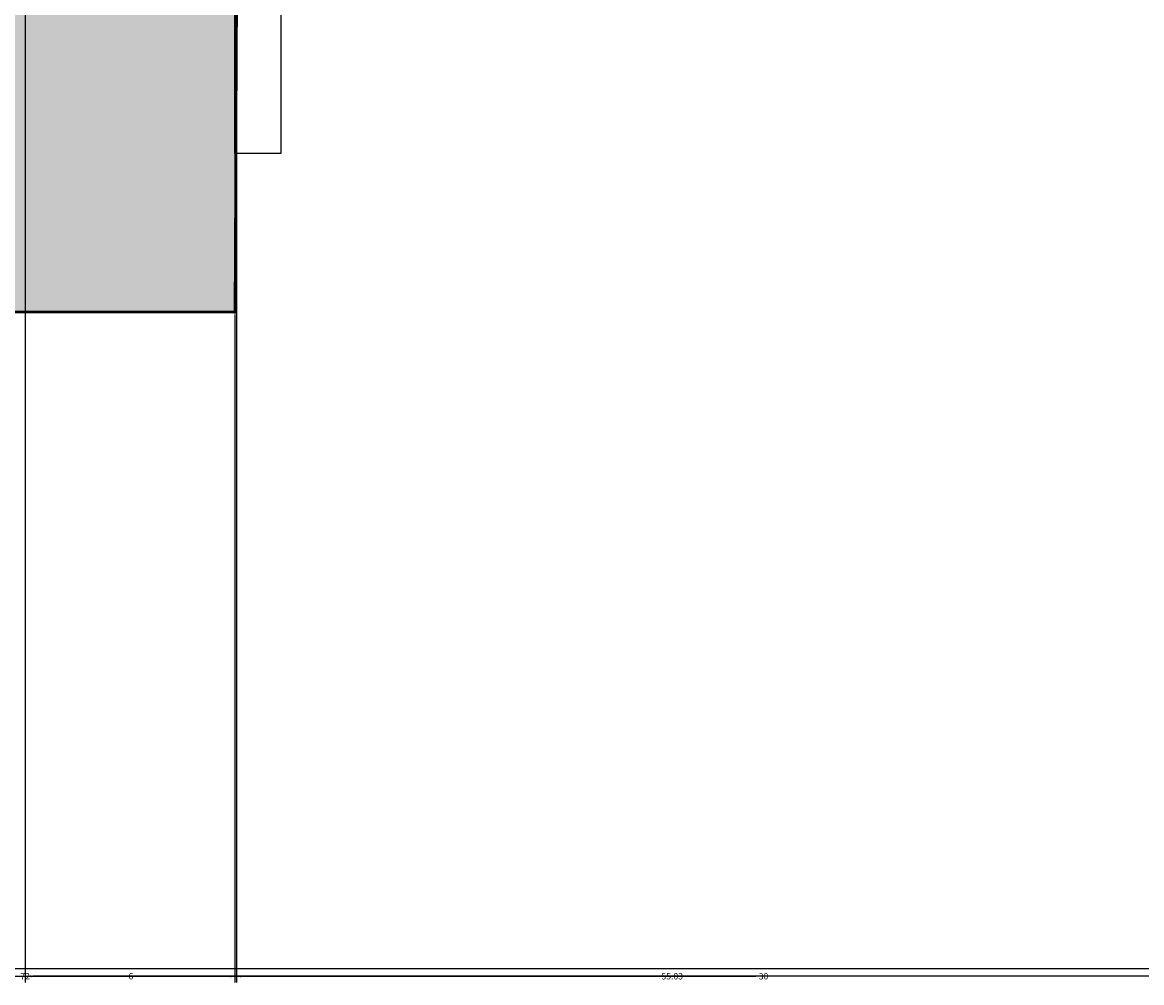
# Model space of a CAD drawing. Units: inches. Extents: x 2231 to 2461, y 2045 to 2455.
# Tile 4 of 95: x 2295 to 2326, y 2045 to 2072. Entities that reach past the tile are written whole.
import ezdxf

# ---------------------------------------------------------------- set-up
doc = ezdxf.new("R2010")
doc.units = ezdxf.units.IN
for name, color, linetype, lineweight in [('A-ANNO-DIMS', 2, 'Continuous', 18), ('A-DOOR', 3, 'Continuous', 25), ('A-WALL', 7, 'Continuous', 50)]:
    doc.layers.add(name, color=color, linetype=linetype, lineweight=lineweight)
doc.layers.add('A-WALL-PATT', color=18, linetype='Continuous', lineweight=13, true_color=0x000000)
doc.styles.get("Standard").update_dxf_attribs({"font": 'arial.ttf'})
doc.dimstyles.get("Standard").update_dxf_attribs({"dimtxt": 0.18, "dimasz": 0.18, "dimexe": 0.18, "dimexo": 0.0625, "dimgap": 0.09, "dimtad": 0, "dimtih": 1, "dimtoh": 1, "dimdec": 4, "dimzin": 0, "dimdsep": 46, "dimtxsty": 'Standard', "dimcen": 0.09, "dimadec": 0, "dimazin": 0, "dimtfac": 1, "dimtdec": 4, "dimtofl": 0, "dimtmove": 0, "dimatfit": 3, "dimfxl": 1, "dimtolj": 1, "dimtzin": 0, "dimarcsym": 0})

# ---------------------------------------------------------------- blocks, each defined once
blk = doc.blocks.new('*U5')
blk.add_line((0, 0), (0, -6))
blk.add_lwpolyline([(0, 0), (0, 40), (1.75, 40), (1.75, 0)], close=True)
blk.add_arc((0, 0), 40, 0, 90)
blk = doc.blocks.new('*D33')
at = {"layer": 'A-ANNO-DIMS', "color": 0, "lineweight": -2, "transparency": 16777216}
for p, q in [((2249.794, 2063.77), (2249.794, 2045.02)), ((2441.794, 2063.77), (2441.794, 2045.02)), ((2249.974, 2045.2), (2345.514, 2045.2)), ((2441.614, 2045.2), (2346.073, 2045.2))]:
    blk.add_line(p, q, dxfattribs=at)
at = {"layer": 'A-ANNO-DIMS', "color": 0, "transparency": 16777216}
for points in [[(2249.974, 2045.23), (2249.974, 2045.17), (2249.794, 2045.2)], [(2441.614, 2045.23), (2441.614, 2045.17), (2441.794, 2045.2)]]:
    blk.add_solid(points, dxfattribs=at)
at = {"layer": 'Defpoints', "color": 0, "transparency": 16777216}
for p in [(2249.794, 2063.833), (2441.794, 2063.833), (2249.794, 2045.2)]:
    blk.add_point(p, dxfattribs=at)
at = {"layer": 'A-ANNO-DIMS', "color": 0, "transparency": 16777216, "insert": (2345.794, 2045.2), "char_height": 0.18, "attachment_point": 5}
blk.add_mtext('\\A1;192', dxfattribs=at)
blk = doc.blocks.new('*D44')
at = {"layer": 'A-ANNO-DIMS', "color": 0, "lineweight": -2, "transparency": 16777216}
for p, q in [((2294.794, 2072.77), (2294.794, 2044.803)), ((2300.794, 2072.77), (2300.794, 2044.803)), ((2294.974, 2044.983), (2297.644, 2044.983)), ((2300.614, 2044.983), (2297.943, 2044.983))]:
    blk.add_line(p, q, dxfattribs=at)
at = {"layer": 'A-ANNO-DIMS', "color": 0, "transparency": 16777216}
for points in [[(2294.974, 2045.013), (2294.974, 2044.953), (2294.794, 2044.983)], [(2300.614, 2045.013), (2300.614, 2044.953), (2300.794, 2044.983)]]:
    blk.add_solid(points, dxfattribs=at)
at = {"layer": 'Defpoints', "color": 0, "transparency": 16777216}
for p in [(2294.794, 2072.833), (2300.794, 2072.833), (2300.794, 2044.983)]:
    blk.add_point(p, dxfattribs=at)
at = {"layer": 'A-ANNO-DIMS', "color": 0, "transparency": 16777216, "insert": (2297.794, 2044.983), "char_height": 0.18, "attachment_point": 5}
blk.add_mtext('\\A1;6', dxfattribs=at)
blk = doc.blocks.new('*D45')
at = {"layer": 'A-ANNO-DIMS', "color": 0, "lineweight": -2, "transparency": 16777216}
for p, q in [((2300.739, 2063.77), (2300.739, 2044.803)), ((2330.74, 2063.77), (2330.74, 2044.803)), ((2300.919, 2044.983), (2315.521, 2044.983)), ((2330.56, 2044.983), (2315.958, 2044.983))]:
    blk.add_line(p, q, dxfattribs=at)
at = {"layer": 'A-ANNO-DIMS', "color": 0, "transparency": 16777216}
for points in [[(2300.919, 2045.013), (2300.919, 2044.953), (2300.739, 2044.983)], [(2330.56, 2045.013), (2330.56, 2044.953), (2330.74, 2044.983)]]:
    blk.add_solid(points, dxfattribs=at)
at = {"layer": 'Defpoints', "color": 0, "transparency": 16777216}
for p in [(2300.739, 2063.833), (2330.74, 2063.833), (2330.74, 2044.983)]:
    blk.add_point(p, dxfattribs=at)
at = {"layer": 'A-ANNO-DIMS', "color": 0, "transparency": 16777216, "insert": (2315.739, 2044.983), "char_height": 0.18, "attachment_point": 5}
blk.add_mtext('\\A1;30', dxfattribs=at)
blk = doc.blocks.new('*D51')
at = {"layer": 'A-ANNO-DIMS', "color": 0, "lineweight": -2, "transparency": 16777216}
for p, q in [((2258.794, 2306.77), (2258.794, 2044.803)), ((2330.794, 2306.77), (2330.794, 2044.803)), ((2258.974, 2044.983), (2294.576, 2044.983)), ((2330.614, 2044.983), (2295.011, 2044.983))]:
    blk.add_line(p, q, dxfattribs=at)
at = {"layer": 'A-ANNO-DIMS', "color": 0, "transparency": 16777216}
for points in [[(2258.974, 2045.013), (2258.974, 2044.953), (2258.794, 2044.983)], [(2330.614, 2045.013), (2330.614, 2044.953), (2330.794, 2044.983)]]:
    blk.add_solid(points, dxfattribs=at)
at = {"layer": 'Defpoints', "color": 0, "transparency": 16777216}
for p in [(2258.794, 2306.833), (2330.794, 2306.833), (2330.794, 2044.983)]:
    blk.add_point(p, dxfattribs=at)
at = {"layer": 'A-ANNO-DIMS', "color": 0, "transparency": 16777216, "insert": (2294.794, 2044.983), "char_height": 0.18, "attachment_point": 5}
blk.add_mtext('\\A1;72', dxfattribs=at)
blk = doc.blocks.new('*D65')
at = {"layer": 'A-ANNO-DIMS', "color": 0, "lineweight": -2, "transparency": 16777216}
for p, q in [((2285.635, 2189.285), (2285.635, 2044.803)), ((2340.667, 2189.285), (2340.667, 2044.803)), ((2285.815, 2044.983), (2312.758, 2044.983)), ((2340.487, 2044.983), (2313.545, 2044.983))]:
    blk.add_line(p, q, dxfattribs=at)
at = {"layer": 'A-ANNO-DIMS', "color": 0, "transparency": 16777216}
for points in [[(2285.815, 2045.013), (2285.815, 2044.953), (2285.635, 2044.983)], [(2340.487, 2045.013), (2340.487, 2044.953), (2340.667, 2044.983)]]:
    blk.add_solid(points, dxfattribs=at)
at = {"layer": 'Defpoints', "color": 0, "transparency": 16777216}
for p in [(2285.635, 2189.348), (2340.667, 2189.348), (2340.667, 2044.983)]:
    blk.add_point(p, dxfattribs=at)
at = {"layer": 'A-ANNO-DIMS', "color": 0, "transparency": 16777216, "insert": (2313.151, 2044.983), "char_height": 0.18, "attachment_point": 5}
blk.add_mtext('\\A1;55.03', dxfattribs=at)

msp = doc.modelspace()

# ---------------------------------------------------------------- hatches: boundary and pattern name
at = {"layer": 'A-WALL-PATT'}
h = msp.add_hatch(color=256, dxfattribs=at)
h.dxf.hatch_style = 1
h.paths.add_polyline_path([(2441.7935, 2269.1535), (2432.7935, 2269.1535), (2432.7935, 2186.8328), (2396.7935, 2186.8328), (2396.7935, 2286.8328), (2394.7935, 2286.8328), (2394.7935, 2186.8328), (2334.7935, 2186.8328), (2334.7935, 2182.8328), (2432.7935, 2182.8328), (2432.7935, 2072.8328), (2416.6639, 2072.8328), (2416.6639, 2063.8328), (2441.7935, 2063.8328)])
h.paths.add_polyline_path([(2368.6639, 2072.8328), (2367.04, 2072.8328), (2330.7942, 2072.8328), (2330.7397, 2063.8328), (2368.6639, 2063.8328)])
h.paths.add_polyline_path([(2300.7392, 2068.3328), (2300.7392, 2072.8328), (2298.7935, 2072.8328), (2294.7935, 2072.8328), (2258.7935, 2072.8328), (2258.7935, 2120.8328), (2294.7935, 2120.8328), (2298.7935, 2120.8328), (2298.7935, 2128.8328), (2294.7935, 2128.8328), (2294.7935, 2124.8328), (2258.7935, 2124.8328), (2258.7935, 2182.8328), (2294.7935, 2182.8328), (2294.7935, 2174.8328), (2298.7935, 2174.8328), (2298.7935, 2182.8328), (2304.7935, 2182.8328), (2304.7935, 2186.8328), (2258.7935, 2186.8328), (2258.7935, 2221.999), (2249.7935, 2221.999), (2249.7935, 2063.8328), (2300.7392, 2063.8328)])
h.paths.add_polyline_path([(2391.9338, 2435.8328), (2333.82, 2435.8328), (2333.82, 2426.8328), (2368.7935, 2426.8328), (2368.7935, 2374.9508), (2368.7935, 2370.8328), (2372.3935, 2370.8328), (2372.7935, 2370.8328), (2372.7935, 2426.8328), (2391.9338, 2426.8328)])
h.paths.add_polyline_path([(2441.7935, 2435.8328), (2415.9338, 2435.8328), (2415.9338, 2426.8328), (2432.7935, 2426.8328), (2432.7935, 2334.8328), (2372.7935, 2334.8328), (2372.7935, 2346.8328), (2368.7935, 2346.8328), (2368.7935, 2306.8328), (2360.7935, 2306.8328), (2360.7935, 2302.8328), (2368.7935, 2302.8328), (2372.7935, 2302.8328), (2372.7935, 2330.8328), (2432.7935, 2330.8328), (2432.7935, 2317.1535), (2441.7935, 2317.1535)])
h.paths.add_polyline_path([(2285.82, 2435.8328), (2249.7935, 2435.8328), (2249.7935, 2269.999), (2258.7935, 2269.999), (2258.7935, 2302.8328), (2318.8168, 2302.8328), (2330.7935, 2302.8328), (2330.7935, 2306.8328), (2258.7935, 2306.8328), (2258.7935, 2426.8328), (2285.82, 2426.8328)])

# ---------------------------------------------------------------- linework, layer by layer
at = {"layer": 'A-WALL'}
msp.add_line((2300.7936, 2072.8328), (2300.739, 2063.7965), dxfattribs=at)
msp.add_lwpolyline([(2300.7392, 2063.8328), (2249.7935, 2063.8328), (2249.7935, 2435.8328), (2441.7935, 2435.8328), (2441.7935, 2063.8328), (2330.7397, 2063.8328)], dxfattribs=at)

# ---------------------------------------------------------------- block references
at = {"layer": 'A-DOOR', "xscale": 0.75, "yscale": 0.75, "zscale": 0.75}
msp.add_blockref('*U5', (2300.7392, 2068.3328), dxfattribs=at)

# ---------------------------------------------------------------- dimensions: what is measured, and where the dimension line sits
at = {"layer": 'A-ANNO-DIMS'}
for base, p1, p2, override, picture, middle in [((2330.7935, 2044.9825), (2258.7935, 2306.8328), (2330.7935, 2306.8328), {"dimdec": 0, "dimlfac": 1, "dimrnd": 0, "dimzin": 0, "dimdsep": 46, "dimlunit": 2}, '*D51', (2294.7935, 2044.9825)), ((2340.6673, 2044.9825), (2285.6353, 2189.3477), (2340.6673, 2189.3477), {"dimdec": 2, "dimlfac": 1, "dimrnd": 0, "dimzin": 0, "dimdsep": 46, "dimlunit": 2}, '*D65', (2313.1513, 2044.9825)), ((2300.7936, 2044.9825), (2294.7935, 2072.8328), (2300.7936, 2072.8328), {"dimdec": 0, "dimlfac": 1, "dimrnd": 0, "dimzin": 0, "dimdsep": 46, "dimlunit": 2}, '*D44', (2297.7936, 2044.9825)), ((2330.7397, 2044.9825), (2300.7392, 2063.8328), (2330.7397, 2063.8328), {"dimdec": 0, "dimlfac": 1, "dimrnd": 0, "dimzin": 0, "dimdsep": 46, "dimlunit": 2}, '*D45', (2315.7395, 2044.9825))]:
    dim = msp.add_linear_dim(base=base, p1=p1, p2=p2, dimstyle='Standard', override=override, dxfattribs=at)
    dim.commit()
    dim.dimension.update_dxf_attribs({"geometry": picture, "text_midpoint": middle})
dim = msp.add_linear_dim(base=(2249.7935, 2045.2003), p1=(2441.7935, 2063.8328), p2=(2249.7935, 2063.8328), angle=180, dimstyle='Standard', override={"dimdec": 0, "dimlfac": 1, "dimrnd": 0, "dimzin": 0, "dimdsep": 46, "dimlunit": 2}, dxfattribs=at)
dim.commit()
dim.dimension.update_dxf_attribs({"geometry": '*D33', "text_midpoint": (2345.7935, 2045.2003)})

doc.saveas('drawing.dxf')
